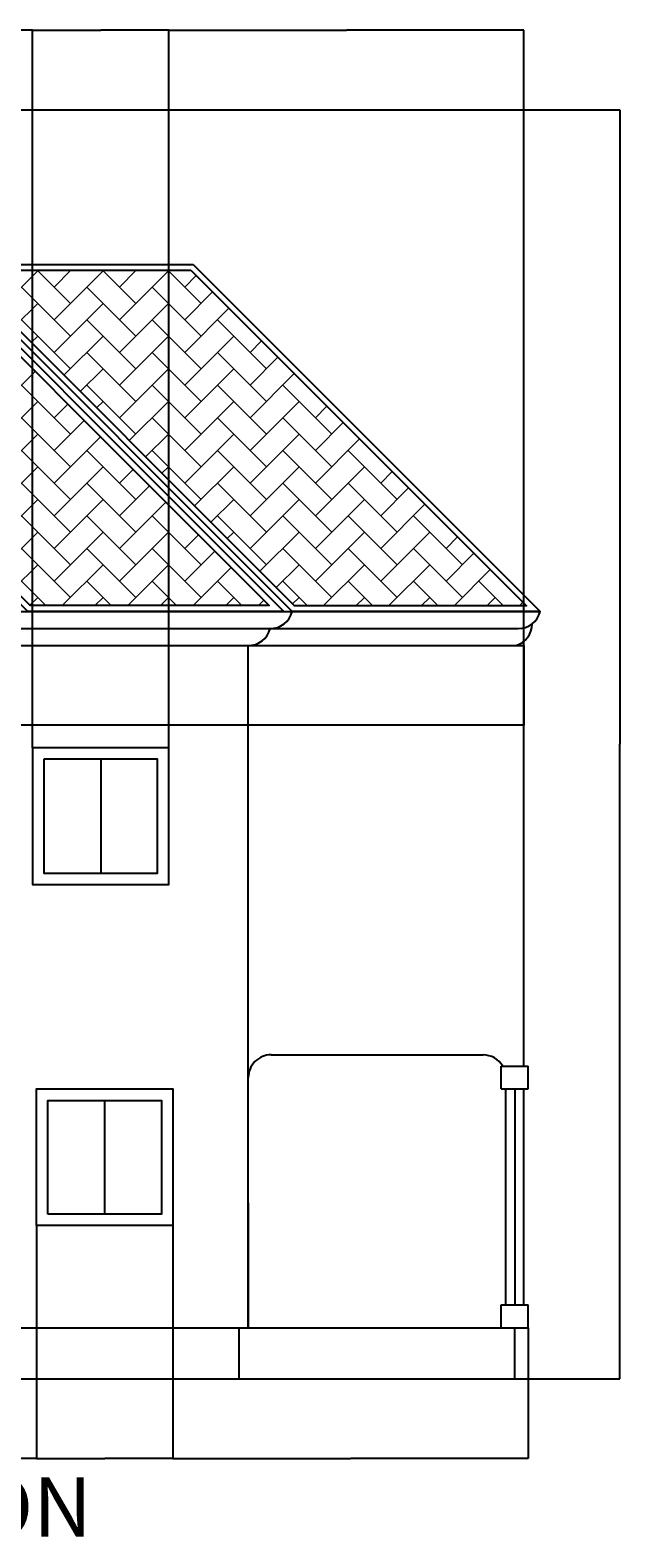
# Model space of a CAD drawing. Units: millimetres. Extents: x 19292 to 100733, y 12374 to 26974.
# Tile 24 of 24: x 95547 to 100733, y 13711 to 26974. Entities that reach past the tile are written whole.
import ezdxf

# ---------------------------------------------------------------- set-up
doc = ezdxf.new("R2010")
doc.units = ezdxf.units.MM
for name, color, linetype, lineweight in [('A-ANNO-DIMS', 2, 'Continuous', 18), ('A-ANNO-TEXT', 7, 'Continuous', 35), ('A-ELEV', 7, 'Continuous', 25), ('A-ELEV-PATT', 8, 'Continuous', 13)]:
    doc.layers.add(name, color=color, linetype=linetype, lineweight=lineweight)
doc.styles.get("Standard").update_dxf_attribs({"font": 'arial.ttf'})
doc.dimstyles.get("Standard").update_dxf_attribs({"dimtxt": 0.18, "dimasz": 0.18, "dimexe": 0.18, "dimexo": 0.0625, "dimgap": 0.09, "dimtad": 0, "dimtih": 1, "dimtoh": 1, "dimdec": 4, "dimzin": 0, "dimdsep": 46, "dimtxsty": 'Standard', "dimcen": 0.09, "dimadec": 0, "dimazin": 0, "dimtfac": 1, "dimtdec": 4, "dimtofl": 0, "dimtmove": 0, "dimatfit": 3, "dimfxl": 1, "dimtolj": 1, "dimtzin": 0, "dimarcsym": 0})

# ---------------------------------------------------------------- blocks, each defined once
blk = doc.blocks.new('WIN-ELEV-1200')
blk.add_line((599.9999832836038, 1100.000156100592), (599.9999832836038, 100.000156100592))
for points in [[(1199.999983283604, 1200.000156100592), (1199.999983283604, 0.0001561005919939), (-1.67163962033e-05, 0.0001561005919939), (-1.67163962033e-05, 1200.000156100592)], [(1099.999983283604, 1100.000156100592), (1099.999983283604, 100.000156100592), (99.9999832836038, 100.000156100592), (99.9999832836038, 1100.000156100592)]]:
    blk.add_lwpolyline(points, close=True)
blk = doc.blocks.new('*D151')
at = {"layer": 'A-ANNO-DIMS', "color": 0, "lineweight": -2, "transparency": 16777216}
for p, q in [((91039.56247500001, 26274.21100900001), (100732.6942110001, 26274.21100900001)), ((100732.5142110001, 26274.03100900001), (100732.5142110001, 20692.2419856378)), ((100732.5142110001, 15110.08915600001), (100732.5142110001, 20691.87817936222)), ((99927.91327500006, 15109.909156), (100732.6942110001, 15109.909156))]:
    blk.add_line(p, q, dxfattribs=at)
at = {"layer": 'A-ANNO-DIMS', "color": 0, "transparency": 16777216}
for points in [[(100732.4842110001, 26274.03100900001), (100732.5442110001, 26274.03100900001), (100732.5142110001, 26274.21100900001)], [(100732.4842110001, 15110.08915600001), (100732.5442110001, 15110.08915600001), (100732.5142110001, 15109.909156)]]:
    blk.add_solid(points, dxfattribs=at)
at = {"layer": 'Defpoints', "color": 0, "transparency": 16777216}
for p in [(91039.49997500001, 26274.21100900001), (100732.5142110001, 26274.21100900001), (99927.85077500006, 15109.909156)]:
    blk.add_point(p, dxfattribs=at)
at = {"layer": 'A-ANNO-DIMS', "color": 0, "transparency": 16777216, "insert": (100732.5142110001, 20692.06008249997), "char_height": 0.18, "attachment_point": 5}
blk.add_mtext('\\A1;11164', dxfattribs=at)
blk = doc.blocks.new('*D158')
at = {"layer": 'A-ANNO-DIMS', "color": 0, "lineweight": -2, "transparency": 16777216}
for p, q in [((95602.426915, 16459.846656), (95602.426915, 14409.716173)), ((94875.223652, 15559.846656), (94875.223652, 14409.716173)), ((94875.403652, 14409.896173), (95238.43323711529, 14409.896173)), ((95602.24691500001, 14409.896173), (95239.21732988473, 14409.896173))]:
    blk.add_line(p, q, dxfattribs=at)
at = {"layer": 'A-ANNO-DIMS', "color": 0, "transparency": 16777216}
for points in [[(94875.403652, 14409.926173), (94875.403652, 14409.866173), (94875.223652, 14409.896173)], [(95602.24691500001, 14409.926173), (95602.24691500001, 14409.866173), (95602.426915, 14409.896173)]]:
    blk.add_solid(points, dxfattribs=at)
at = {"layer": 'Defpoints', "color": 0, "transparency": 16777216}
for p in [(95602.426915, 16459.909156), (94875.223652, 15559.909156), (95602.426915, 14409.896173)]:
    blk.add_point(p, dxfattribs=at)
at = {"layer": 'A-ANNO-DIMS', "color": 0, "transparency": 16777216, "insert": (95238.8252835, 14409.896173), "char_height": 0.18, "attachment_point": 5}
blk.add_mtext('\\A1;727.2', dxfattribs=at)
blk = doc.blocks.new('*D159')
at = {"layer": 'A-ANNO-DIMS', "color": 0, "lineweight": -2, "transparency": 16777216}
for p, q in [((95602.426915, 16459.846656), (95602.426915, 14409.716173)), ((96802.426915, 16459.846656), (96802.426915, 14409.716173)), ((95602.606915, 14409.896173), (96202.0769218213, 14409.896173)), ((96802.24691500001, 14409.896173), (96202.77690817873, 14409.896173))]:
    blk.add_line(p, q, dxfattribs=at)
at = {"layer": 'A-ANNO-DIMS', "color": 0, "transparency": 16777216}
for points in [[(95602.606915, 14409.926173), (95602.606915, 14409.866173), (95602.426915, 14409.896173)], [(96802.24691500001, 14409.926173), (96802.24691500001, 14409.866173), (96802.426915, 14409.896173)]]:
    blk.add_solid(points, dxfattribs=at)
at = {"layer": 'Defpoints', "color": 0, "transparency": 16777216}
for p in [(95602.426915, 16459.909156), (96802.426915, 16459.909156), (96802.426915, 14409.896173)]:
    blk.add_point(p, dxfattribs=at)
at = {"layer": 'A-ANNO-DIMS', "color": 0, "transparency": 16777216, "insert": (96202.426915, 14409.896173), "char_height": 0.18, "attachment_point": 5}
blk.add_mtext('\\A1;1200', dxfattribs=at)
blk = doc.blocks.new('*D160')
at = {"layer": 'A-ANNO-DIMS', "color": 0, "lineweight": -2, "transparency": 16777216}
for p, q in [((96802.426915, 16459.846656), (96802.426915, 14409.716173)), ((99927.850775, 15559.846656), (99927.850775, 14409.716173)), ((96802.606915, 14409.896173), (98364.67564581856, 14409.896173)), ((99927.670775, 14409.896173), (98365.60204418146, 14409.896173))]:
    blk.add_line(p, q, dxfattribs=at)
at = {"layer": 'A-ANNO-DIMS', "color": 0, "transparency": 16777216}
for points in [[(96802.606915, 14409.926173), (96802.606915, 14409.866173), (96802.426915, 14409.896173)], [(99927.670775, 14409.926173), (99927.670775, 14409.866173), (99927.850775, 14409.896173)]]:
    blk.add_solid(points, dxfattribs=at)
at = {"layer": 'Defpoints', "color": 0, "transparency": 16777216}
for p in [(96802.426915, 16459.909156), (99927.850775, 15559.909156), (99927.850775, 14409.896173)]:
    blk.add_point(p, dxfattribs=at)
at = {"layer": 'A-ANNO-DIMS', "color": 0, "transparency": 16777216, "insert": (98365.13884500002, 14409.896173), "char_height": 0.18, "attachment_point": 5}
blk.add_mtext('\\A1;3125.4', dxfattribs=at)
blk = doc.blocks.new('*D167')
at = {"layer": 'A-ANNO-DIMS', "color": 0, "lineweight": -2, "transparency": 16777216}
for p, q in [((94913.341746, 20659.971656), (94913.341746, 26974.391009)), ((94913.52174600001, 26974.211009), (95240.02142701363, 26974.211009)), ((95567.099048, 26974.211009), (95240.59936698635, 26974.211009)), ((95567.279048, 20659.971656), (95567.279048, 26974.391009))]:
    blk.add_line(p, q, dxfattribs=at)
at = {"layer": 'A-ANNO-DIMS', "color": 0, "transparency": 16777216}
for points in [[(94913.52174600001, 26974.241009), (94913.52174600001, 26974.181009), (94913.341746, 26974.211009)], [(95567.099048, 26974.241009), (95567.099048, 26974.181009), (95567.279048, 26974.211009)]]:
    blk.add_solid(points, dxfattribs=at)
at = {"layer": 'Defpoints', "color": 0, "transparency": 16777216}
for p in [(95567.279048, 26974.211009), (94913.341746, 20659.909156), (95567.279048, 20659.909156)]:
    blk.add_point(p, dxfattribs=at)
at = {"layer": 'A-ANNO-DIMS', "color": 0, "transparency": 16777216, "insert": (95240.310397, 26974.211009), "char_height": 0.18, "attachment_point": 5}
blk.add_mtext('\\A1;654', dxfattribs=at)
blk = doc.blocks.new('*D168')
at = {"layer": 'A-ANNO-DIMS', "color": 0, "lineweight": -2, "transparency": 16777216}
for p, q in [((95567.279048, 20659.971656), (95567.279048, 26974.391009)), ((95567.45904799999, 26974.211009), (96166.92905482127, 26974.211009)), ((96767.099048, 26974.211009), (96167.6290411787, 26974.211009)), ((96767.279048, 20659.971656), (96767.279048, 26974.391009))]:
    blk.add_line(p, q, dxfattribs=at)
at = {"layer": 'A-ANNO-DIMS', "color": 0, "transparency": 16777216}
for points in [[(95567.45904799999, 26974.241009), (95567.45904799999, 26974.181009), (95567.279048, 26974.211009)], [(96767.099048, 26974.241009), (96767.099048, 26974.181009), (96767.279048, 26974.211009)]]:
    blk.add_solid(points, dxfattribs=at)
at = {"layer": 'Defpoints', "color": 0, "transparency": 16777216}
for p in [(96767.279048, 26974.211009), (95567.279048, 20659.909156), (96767.279048, 20659.909156)]:
    blk.add_point(p, dxfattribs=at)
at = {"layer": 'A-ANNO-DIMS', "color": 0, "transparency": 16777216, "insert": (96167.279048, 26974.211009), "char_height": 0.18, "attachment_point": 5}
blk.add_mtext('\\A1;1200', dxfattribs=at)
blk = doc.blocks.new('*D169')
at = {"layer": 'A-ANNO-DIMS', "color": 0, "lineweight": -2, "transparency": 16777216}
for p, q in [((96767.279048, 20659.971656), (96767.279048, 26974.391009)), ((96767.45904799998, 26974.211009), (98327.60853986084, 26974.211009)), ((99888.685044, 26974.211009), (98328.53555213915, 26974.211009)), ((99888.865044, 21559.971656), (99888.865044, 26974.391009))]:
    blk.add_line(p, q, dxfattribs=at)
at = {"layer": 'A-ANNO-DIMS', "color": 0, "transparency": 16777216}
for points in [[(96767.45904799998, 26974.241009), (96767.45904799998, 26974.181009), (96767.279048, 26974.211009)], [(99888.685044, 26974.241009), (99888.685044, 26974.181009), (99888.865044, 26974.211009)]]:
    blk.add_solid(points, dxfattribs=at)
at = {"layer": 'Defpoints', "color": 0, "transparency": 16777216}
for p in [(99888.865044, 26974.211009), (99888.865044, 21559.909156), (96767.279048, 20659.909156)]:
    blk.add_point(p, dxfattribs=at)
at = {"layer": 'A-ANNO-DIMS', "color": 0, "transparency": 16777216, "insert": (98328.07204599999, 26974.211009), "char_height": 0.18, "attachment_point": 5}
blk.add_mtext('\\A1;3121.6', dxfattribs=at)
blk = doc.blocks.new('*D170')
at = {"layer": 'A-ANNO-DIMS', "color": 0, "lineweight": -2, "transparency": 16777216}
for p, q in [((86437.814258, 21559.846656), (86437.814258, 20859.729156)), ((99888.865044, 21559.846656), (99888.865044, 20859.729156)), ((86437.99425799999, 20859.909156), (93162.93679970397, 20859.909156)), ((99888.685044, 20859.909156), (93163.74250229605, 20859.909156))]:
    blk.add_line(p, q, dxfattribs=at)
at = {"layer": 'A-ANNO-DIMS', "color": 0, "transparency": 16777216}
for points in [[(86437.99425799999, 20859.939156), (86437.99425799999, 20859.879156), (86437.814258, 20859.909156)], [(99888.685044, 20859.939156), (99888.685044, 20859.879156), (99888.865044, 20859.909156)]]:
    blk.add_solid(points, dxfattribs=at)
at = {"layer": 'Defpoints', "color": 0, "transparency": 16777216}
for p in [(86437.814258, 21559.909156), (99888.865044, 21559.909156), (86437.814258, 20859.909156)]:
    blk.add_point(p, dxfattribs=at)
at = {"layer": 'A-ANNO-DIMS', "color": 0, "transparency": 16777216, "insert": (93163.339651, 20859.909156), "char_height": 0.18, "attachment_point": 5}
blk.add_mtext('\\A1;13451', dxfattribs=at)

msp = doc.modelspace()

# ---------------------------------------------------------------- hatches: boundary and pattern name
at = {"layer": 'A-ELEV-PATT'}
h = msp.add_hatch(dxfattribs=at)
h.set_pattern_fill('AR-HBONE', color=256, scale=2)
h.set_pattern_definition([(45, (-15742.66734838602, 1.819e-12), (0, 287.3681958742129), [609.6, -203.2]), (135, (-15598.98334838602, 143.6840000000018), (2.84e-14, 287.3681958742129), [609.6, -203.2])])
h.paths.add_polyline_path([(87735.48117691663, 23052.98438420805), (87536.44885016952, 23052.98438420805), (86378.42981350586, 21894.96534754441), (86578.07896417224, 21895.58217146364)])
h.paths.add_polyline_path([(91039.49997476467, 26192.70967510026), (86764.32960140108, 21917.5393017367), (95314.67034812817, 21917.5393017367)])
h.paths.add_polyline_path([(93872.96419886049, 25688.93910166301), (91772.21995210611, 25688.939101663), (95547.96497158404, 21913.19408218505), (97648.70921833848, 21913.19408218505)])
h.paths.add_polyline_path([(96958.92150424178, 24862.64804519888), (94918.01694600363, 24862.64804519888), (97871.17317701879, 21909.49181418373), (99911.74658381855, 21909.82296562213)])

# ---------------------------------------------------------------- linework, layer by layer
at = {"layer": 'A-ELEV'}
for p, q in [((86294.16509073348, 21859.90915610059), (100032.5142111294, 21859.90915610059)), ((99888.8650438191, 21859.86047104414), (99888.8650438191, 21859.90915610059)), ((86487.81425804386, 21709.9091561006), (99838.86504381908, 21709.90915610059)), ((86437.81425804387, 21559.90915610059), (99888.8650438191, 21559.90915610059)), ((97463.34174630335, 15559.90915610059), (97463.34174630335, 21559.90915610059)), ((99888.8650438191, 18559.90915610059), (99888.8650438191, 21559.90915610059)), ((99887.85077479901, 17859.90915610059), (99887.85077479901, 18559.90915610059)), ((97665.15619167511, 17959.90915610059), (99529.39913993001, 17959.90915610059)), ((99689.39913992997, 17859.90915610059), (99927.850774799, 17859.90915610059)), ((99689.39913992997, 17659.90915610059), (99689.39913992997, 17859.90915610059)), ((99689.39913993001, 17659.90915610059), (99689.39913993001, 17859.90915610059)), ((99927.85077479901, 17659.90915610059), (99927.85077479901, 17859.90915610059)), ((99927.85077479901, 17659.90915610059), (99927.85077479901, 17859.90915610059)), ((97465.5132127888, 15559.90915610059), (97465.15619430869, 17759.87669939672)), ((99689.39913992997, 17659.90915610059), (99927.850774799, 17659.90915610059)), ((99729.39913993001, 15759.90915610059), (99729.39913993001, 17659.90915610059)), ((99729.39913993001, 15759.90915610059), (99729.39913993001, 17659.90915610059)), ((99808.62495736449, 17659.90915610059), (99808.6249573645, 15759.90915610059)), ((99887.85077479901, 15759.90915610059), (99887.85077479901, 17659.90915610059)), ((99887.85077479901, 15759.90915610059), (99887.85077479901, 17659.90915610059)), ((99689.39913993001, 15559.90915610059), (99689.39913993001, 15759.90915610059)), ((99689.39913993001, 15559.90915610059), (99689.39913993001, 15759.90915610059)), ((99689.39913993001, 15759.90915610059), (99927.85077479901, 15759.90915610059)), ((99927.85077479901, 15559.90915610059), (99927.85077479901, 15759.90915610059)), ((99927.85077479901, 15559.90915610059), (99927.85077479901, 15759.90915610059)), ((86437.81425804387, 15559.90915610059), (99927.85077479901, 15559.90915610059)), ((97385.58624142692, 15109.89617341904), (97385.51321173536, 15559.90915610059)), ((99807.850774799, 15109.90915610059), (99807.850774799, 15559.90915610059)), ((86437.81425804387, 15109.90915610059), (99927.85077479901, 15109.90915610059))]:
    msp.add_line(p, q, dxfattribs=at)
for points in [[(93895.19421929128, 25742.60711847879), (97778.27527240079, 21859.52606536928), (95525.73495115327, 21859.52606536928), (91642.65389804375, 25742.60711847878)], [(96979.45793317242, 24912.22737044603), (100031.422242509, 21860.26306110946), (97850.6400809241, 21859.90915610059), (94798.32186657867, 24912.22737044603), (96979.45793317242, 24912.22737044603)]]:
    msp.add_lwpolyline(points, dxfattribs=at)
for points in [[(93872.96419886049, 25688.93910166301), (97648.70921833848, 21913.19408218505), (95547.96497158404, 21913.19408218505), (91772.21995210611, 25688.939101663)], [(96958.92150424178, 24862.64804519888), (99911.74658381855, 21909.82296562213), (97871.17317701879, 21909.49181418373), (94918.01694600363, 24862.64804519888)]]:
    msp.add_lwpolyline(points, close=True, dxfattribs=at)
for centre, start, end in [((97656.99091361373, 21909.90915610059), 270, 345.5224878140609), ((99761.33953095818, 21751.79527309215), 286.3763195261408, 0), ((99838.86504381908, 21909.90915610059), 270, 345.5224878140591), ((97463.34174630335, 21759.90915610059), 270, 345.5224878140829), ((97665.15619167511, 17759.90915610059), 90, 180.0092981607568), ((99529.39913993001, 17759.90915610059), 30.00000000009106, 90)]:
    msp.add_arc(centre, 200, start, end, dxfattribs=at)

# ---------------------------------------------------------------- block references
at = {"layer": 'A-ELEV', "extrusion": (0, 0, -1), "zscale": -1}
msp.add_blockref('WIN-ELEV-1200', (-96767.27903097718, 19459.909), dxfattribs=at)
at = {"layer": 'A-ELEV', "rotation": 180}
msp.add_blockref('WIN-ELEV-1200', (96802.42689870072, 17659.90931220118), dxfattribs=at)

# ---------------------------------------------------------------- texts
at = {"layer": 'A-ANNO-TEXT'}
msp.add_text('APPROACH ELEVATION', height=523.2684807306957, dxfattribs=at).set_placement((88444.08516921198, 13720.60677981616))

# ---------------------------------------------------------------- dimensions: what is measured, and where the dimension line sits
at = {"layer": 'A-ANNO-DIMS'}
for base, p1, p2, override, picture, middle in [((95567.279048, 26974.211009), (94913.341746, 20659.909156), (95567.279048, 20659.909156), {"dimdec": 0, "dimlfac": 1, "dimrnd": 0, "dimzin": 0, "dimdsep": 46, "dimlunit": 2}, '*D167', (95240.310397, 26974.211009)), ((96767.279048, 26974.211009), (95567.279048, 20659.909156), (96767.279048, 20659.909156), {"dimdec": 0, "dimlfac": 1, "dimrnd": 0, "dimzin": 0, "dimdsep": 46, "dimlunit": 2}, '*D168', (96167.279048, 26974.211009)), ((99888.865044, 26974.211009), (96767.279048, 20659.909156), (99888.865044, 21559.909156), {"dimdec": 1, "dimlfac": 1, "dimrnd": 0, "dimzin": 0, "dimdsep": 46, "dimlunit": 2}, '*D169', (98328.07204599999, 26974.211009)), ((95602.426915, 14409.896173), (94875.223652, 15559.909156), (95602.426915, 16459.909156), {"dimdec": 1, "dimlfac": 1, "dimrnd": 0, "dimzin": 0, "dimdsep": 46, "dimlunit": 2}, '*D158', (95238.8252835, 14409.896173)), ((96802.426915, 14409.896173), (95602.426915, 16459.909156), (96802.426915, 16459.909156), {"dimdec": 0, "dimlfac": 1, "dimrnd": 0, "dimzin": 0, "dimdsep": 46, "dimlunit": 2}, '*D159', (96202.426915, 14409.896173)), ((99927.850775, 14409.896173), (96802.426915, 16459.909156), (99927.850775, 15559.909156), {"dimdec": 1, "dimlfac": 1, "dimrnd": 0, "dimzin": 0, "dimdsep": 46, "dimlunit": 2}, '*D160', (98365.13884500002, 14409.896173))]:
    dim = msp.add_linear_dim(base=base, p1=p1, p2=p2, dimstyle='Standard', override=override, dxfattribs=at)
    dim.commit()
    dim.dimension.update_dxf_attribs({"geometry": picture, "text_midpoint": middle})
for base, p1, p2, angle, picture, middle in [((100732.5142110001, 26274.21100900001), (99927.850775, 15109.909156), (91039.499975, 26274.211009), 90, '*D151', (100732.5142110001, 20692.06008249997)), ((86437.814258, 20859.909156), (99888.865044, 21559.909156), (86437.814258, 21559.909156), 180, '*D170', (93163.339651, 20859.909156))]:
    dim = msp.add_linear_dim(base=base, p1=p1, p2=p2, angle=angle, dimstyle='Standard', override={"dimdec": 0, "dimlfac": 1, "dimrnd": 0, "dimzin": 0, "dimdsep": 46, "dimlunit": 2}, dxfattribs=at)
    dim.commit()
    dim.dimension.update_dxf_attribs({"geometry": picture, "text_midpoint": middle})

doc.saveas('drawing.dxf')
